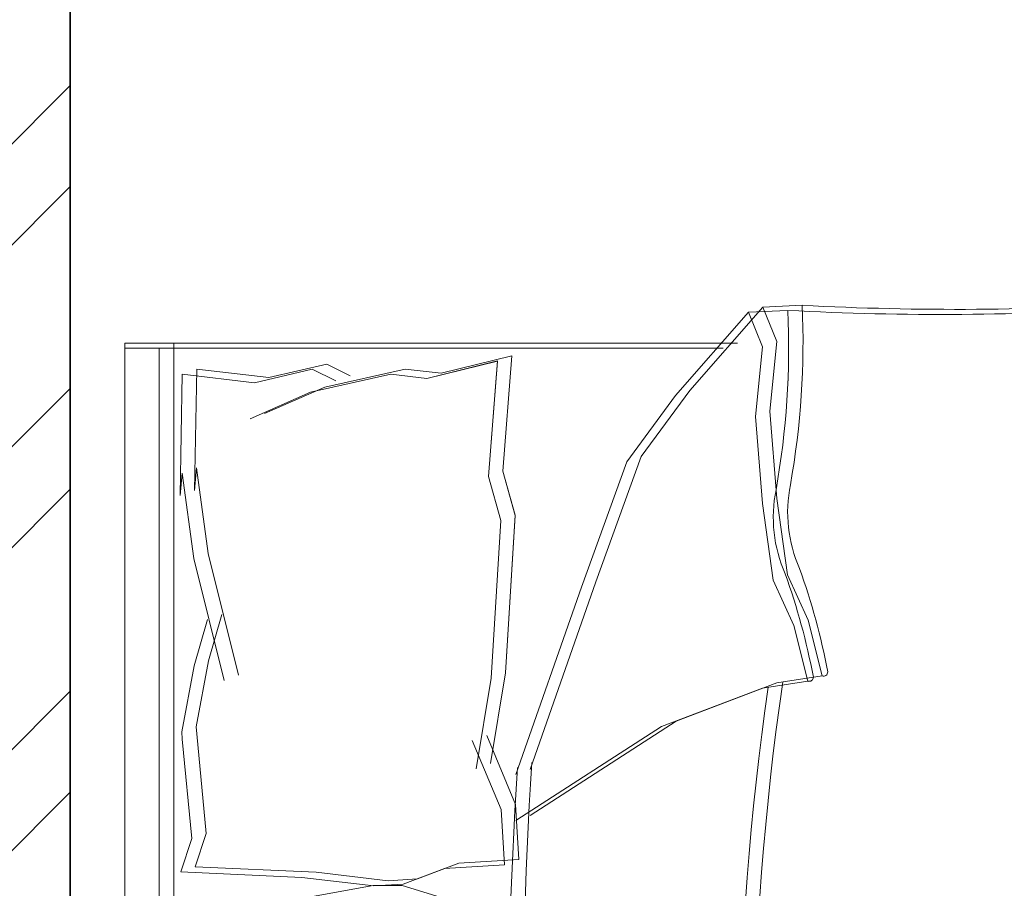
# Model space of a CAD drawing. Units: inches. Extents: x 2168 to 3056, y 1130 to 2629.
# Tile 27 of 42: x 2462 to 2505, y 2347 to 2386. Entities that reach past the tile are written whole.
import ezdxf

# ---------------------------------------------------------------- set-up
doc = ezdxf.new("R2010")
doc.units = ezdxf.units.IN
doc.layers.add('A-FURN', color=8, linetype='Continuous', lineweight=13)
doc.layers.add('A-WALL', color=7, linetype='Continuous', lineweight=35)
doc.layers.add('A-WALL-PATT', color=143, linetype='Continuous', lineweight=13, true_color=0x7aafdf)

# ---------------------------------------------------------------- blocks, each defined once
blk = doc.blocks.new('BED-DOUBLE')
for p, q in [((28.385, 53.096), (25.135, 49.391)), ((28.385, 53.096), (25.135, 49.391)), ((30.13, 53.176), (28.385, 53.096, 3.871)), ((30.13, 53.175), (28.385, 53.096, 3.871)), ((29.005, 51.559), (28.385, 53.096)), ((29.005, 51.559), (28.385, 53.096)), ((27.746, 52.868), (24.496, 49.162)), ((27.746, 52.868), (24.496, 49.162)), ((29.491, 52.947), (27.746, 52.868, 3.871)), ((29.491, 52.947), (27.746, 52.868, 3.871)), ((28.365, 51.331), (27.746, 52.868)), ((28.365, 51.33), (27.746, 52.868)), ((0, 51.494), (0.64, 51.494)), ((0, 3.475), (0, 51.494)), ((0, 51.266), (26.61, 51.266)), ((0, 51.265), (26.61, 51.265)), ((0.64, 51.494), (27.249, 51.494)), ((0.64, 51.494), (27.249, 51.494)), ((1.534, 3.475), (1.534, 51.266)), ((1.534, 3.475), (1.534, 51.265)), ((2.173, 3.704), (2.173, 51.494)), ((2.173, 3.703), (2.173, 51.494)), ((28.056, 48.233), (28.365, 51.331)), ((28.056, 48.233), (28.365, 51.33)), ((28.695, 48.462), (29.005, 51.559)), ((28.695, 48.461), (29.005, 51.559)), ((17.212, 50.927), (14.074, 50.151)), ((17.212, 50.927), (14.074, 50.151)), ((16.809, 45.795), (17.212, 50.927)), ((16.809, 45.795), (17.212, 50.927)), ((6.407, 49.962), (8.978, 50.557)), ((6.407, 49.962), (8.978, 50.557)), ((8.978, 50.557), (10.024, 50.043)), ((8.978, 50.557), (10.024, 50.043)), ((16.573, 50.699), (13.434, 49.923)), ((16.573, 50.698), (13.434, 49.923)), ((16.169, 45.567), (16.573, 50.699)), ((16.169, 45.566), (16.573, 50.698)), ((2.557, 50.112), (2.46, 44.71)), ((2.557, 50.112), (2.46, 44.71)), ((2.557, 50.112), (5.768, 49.734)), ((2.557, 50.112), (5.768, 49.733)), ((3.197, 50.341), (3.1, 44.938)), ((3.197, 50.34), (3.1, 44.938)), ((3.197, 50.341), (6.407, 49.962)), ((3.197, 50.34), (6.407, 49.962)), ((5.768, 49.734), (8.339, 50.329)), ((5.768, 49.733), (8.339, 50.328)), ((11.829, 50.112), (8.257, 49.31)), ((11.829, 50.112), (8.257, 49.309)), ((8.339, 50.329), (9.385, 49.815)), ((8.339, 50.328), (9.385, 49.814)), ((12.468, 50.341), (8.897, 49.538)), ((12.468, 50.34), (8.897, 49.538)), ((13.434, 49.923), (11.829, 50.112)), ((13.434, 49.923), (11.829, 50.112)), ((14.074, 50.151), (12.468, 50.341)), ((14.074, 50.151), (12.468, 50.34)), ((8.897, 49.538), (6.218, 48.357)), ((8.897, 49.538), (6.218, 48.357)), ((8.257, 49.31), (5.579, 48.128)), ((8.257, 49.309), (5.579, 48.128)), ((24.496, 49.162), (22.329, 46.22)), ((24.496, 49.162), (22.329, 46.22)), ((25.135, 49.391), (22.968, 46.448)), ((25.135, 49.391), (22.968, 46.448)), ((28.365, 44.361), (28.056, 48.233)), ((28.365, 44.361), (28.056, 48.233)), ((29.005, 44.59), (28.695, 48.462)), ((29.005, 44.589), (28.695, 48.461)), ((22.968, 46.448), (20.956, 40.873)), ((22.968, 46.448), (20.956, 40.873)), ((22.329, 46.22), (20.317, 40.644)), ((22.329, 46.22), (20.317, 40.644)), ((2.46, 44.71), (2.543, 45.713)), ((2.46, 44.71), (2.543, 45.712)), ((2.543, 45.713), (3.07, 41.915)), ((2.543, 45.712), (3.07, 41.914)), ((3.1, 44.938), (3.182, 45.941)), ((3.1, 44.938), (3.182, 45.941)), ((3.182, 45.941), (3.709, 42.143)), ((3.182, 45.941), (3.709, 42.143)), ((16.727, 43.606), (16.169, 45.567)), ((16.727, 43.606), (16.169, 45.566)), ((17.366, 43.835), (16.809, 45.795)), ((17.366, 43.834), (16.809, 45.795)), ((28.83, 40.954), (28.365, 44.361)), ((28.83, 40.954), (28.365, 44.361)), ((29.469, 41.183), (29.005, 44.59)), ((29.469, 41.182), (29.005, 44.589)), ((16.935, 36.825), (17.366, 43.835)), ((16.935, 36.824), (17.366, 43.834)), ((16.295, 36.596), (16.727, 43.606)), ((16.295, 36.596), (16.727, 43.606)), ((3.709, 42.143), (5.062, 36.724)), ((3.709, 42.143), (5.062, 36.723)), ((3.07, 41.915), (4.422, 36.495)), ((3.07, 41.914), (4.422, 36.495)), ((30.398, 39.169), (29.469, 41.183)), ((30.398, 39.169), (29.469, 41.182)), ((20.956, 40.873), (18.023, 32.535)), ((20.956, 40.873), (18.023, 32.534)), ((29.758, 38.941), (28.83, 40.954)), ((29.758, 38.941), (28.83, 40.954)), ((20.317, 40.644), (17.384, 32.306)), ((20.317, 40.644), (17.384, 32.306)), ((4.313, 39.429), (3.718, 37.364)), ((4.313, 39.429), (3.718, 37.364)), ((3.674, 39.2), (3.079, 37.136)), ((3.674, 39.2), (3.079, 37.135)), ((31.017, 36.691), (30.398, 39.169)), ((31.017, 36.691), (30.398, 39.169)), ((30.377, 36.463), (29.758, 38.941)), ((30.377, 36.463), (29.758, 38.941)), ((3.718, 37.364), (3.177, 34.433)), ((3.718, 37.364), (3.177, 34.433)), ((3.079, 37.136), (2.537, 34.205)), ((3.079, 37.135), (2.537, 34.205)), ((16.268, 32.793), (16.935, 36.825)), ((16.268, 32.793), (16.935, 36.824)), ((15.629, 32.564), (16.295, 36.596)), ((15.629, 32.564), (16.295, 36.596)), ((24.516, 34.678), (29.005, 36.381)), ((24.516, 34.678), (29.005, 36.381)), ((28.365, 36.153), (30.377, 36.463)), ((28.365, 36.153), (30.377, 36.463)), ((29.005, 36.381), (31.017, 36.691)), ((29.005, 36.381), (31.017, 36.691)), ((23.877, 34.45), (28.365, 36.153)), ((23.877, 34.449), (28.365, 36.153)), ((18.023, 30.488), (24.516, 34.678)), ((18.023, 30.488), (24.516, 34.678)), ((2.537, 34.205), (2.557, 33.884)), ((2.537, 34.205), (2.557, 33.884)), ((3.177, 34.433), (3.197, 34.112)), ((3.177, 34.433), (3.197, 34.112)), ((17.384, 30.259), (23.877, 34.45)), ((17.384, 30.259), (23.877, 34.449)), ((2.557, 33.884), (2.979, 29.456)), ((2.557, 33.884), (2.979, 29.456)), ((3.197, 34.112), (3.618, 29.684)), ((3.197, 34.112), (3.618, 29.684)), ((16.74, 30.751), (15.455, 33.821)), ((16.74, 30.75), (15.455, 33.821)), ((17.379, 30.979), (16.094, 34.049)), ((17.379, 30.979), (16.094, 34.049)), ((16.893, 28.298), (16.74, 30.751)), ((16.893, 28.298), (16.74, 30.75)), ((17.532, 28.526), (17.379, 30.979)), ((17.532, 28.526), (17.379, 30.979)), ((2.979, 29.456), (2.492, 27.977)), ((2.979, 29.456), (2.492, 27.977)), ((3.618, 29.684), (3.131, 28.206)), ((3.618, 29.684), (3.131, 28.205)), ((14.856, 28.359), (17.532, 28.526)), ((14.856, 28.359), (17.532, 28.526)), ((3.131, 28.206), (8.507, 27.962)), ((3.131, 28.205), (8.507, 27.962)), ((12.377, 27.436), (14.217, 28.131)), ((12.377, 27.436), (14.217, 28.13)), ((13.016, 27.665), (14.856, 28.359)), ((13.016, 27.664), (14.856, 28.359)), ((14.217, 28.131), (16.893, 28.298)), ((14.217, 28.13), (16.893, 28.298)), ((2.492, 27.977), (7.867, 27.734)), ((2.492, 27.977), (7.867, 27.733)), ((7.867, 27.734), (11.078, 27.355)), ((7.867, 27.733), (11.078, 27.355)), ((8.507, 27.962), (11.718, 27.583)), ((8.507, 27.962), (11.718, 27.583)), ((11.718, 27.583), (13.016, 27.665)), ((11.718, 27.583), (13.016, 27.664)), ((7.86, 26.789), (11.04, 27.368)), ((7.86, 26.789), (11.04, 27.367)), ((11.04, 27.368), (12.342, 27.368)), ((11.04, 27.367), (12.342, 27.367)), ((11.078, 27.355), (12.377, 27.436)), ((11.078, 27.355), (12.377, 27.436)), ((12.342, 27.368), (14.221, 26.789)), ((12.342, 27.367), (14.221, 26.789))]:
    blk.add_line(p, q)
for centre, radius, start, end in [((36.315, 182.266), 129.499, 266.97912, 273.83645), ((36.315, 182.266), 129.499, 266.97912, 273.83645), ((-6.017, 51.556), 36.183, 349.8763, 2.5657), ((-6.017, 51.556), 36.183, 349.8763, 2.5657), ((36.955, 182.494), 129.499, 266.97912, 273.83645), ((36.955, 182.494), 129.499, 266.97912, 273.83645), ((-6.656, 51.328), 36.183, 349.8763, 2.5657), ((-6.656, 51.327), 36.183, 349.8763, 2.5657), ((35.706, 43.972), 6.224, 168.6608, 203.7384), ((35.706, 43.972), 6.224, 168.6608, 203.7384), ((35.067, 43.744), 6.224, 168.6608, 203.7384), ((35.067, 43.743), 6.224, 168.6608, 203.7384), ((1.482, 31.154), 29.654, 10.6617, 19.8806), ((1.482, 31.154), 29.654, 10.6617, 19.8806), ((2.122, 31.382), 29.654, 10.6617, 19.8806), ((2.122, 31.382), 29.654, 10.6617, 19.8806), ((31.079, 36.865), 0.185, 250.2464, 1.1377), ((31.079, 36.865), 0.185, 250.2464, 1.1377), ((156.956, 17.984), 129.02, 171.78449, 186.90062), ((156.956, 17.984), 129.02, 171.78449, 186.90062), ((30.44, 36.637), 0.185, 250.2464, 1.1377), ((30.44, 36.636), 0.185, 250.2464, 1.1377), ((156.317, 17.756), 129.02, 171.78449, 186.90062), ((156.317, 17.756), 129.02, 171.78449, 186.90062), ((182.053, 21.359), 164.969, 176.08655, 186.78213), ((182.053, 21.359), 164.969, 176.08655, 186.78213), ((182.692, 21.587), 164.969, 176.08655, 186.78213), ((182.692, 21.587), 164.969, 176.08655, 186.78213)]:
    blk.add_arc(centre, radius, start, end)

msp = doc.modelspace()

# ---------------------------------------------------------------- hatches: boundary and pattern name
at = {"layer": 'A-WALL-PATT'}
h = msp.add_hatch(dxfattribs=at)
h.set_pattern_fill('ANSI32', color=256)
h.paths.add_polyline_path([(2463.796, 2409.389), (2467.387, 2409.389), (2467.387, 2413.889), (2454.768, 2413.889), (2454.768, 2411.639), (2454.768, 2409.389), (2459.296, 2409.389), (2459.296, 2265.389), (2455.644, 2265.389), (2455.644, 2260.889), (2467.349, 2260.889), (2467.349, 2263.139), (2467.349, 2265.389), (2463.796, 2265.389)])
h.paths.add_polyline_path([(2431.596, 2413.889), (2409.647, 2413.889), (2409.647, 2409.389), (2431.596, 2409.389), (2431.596, 2411.639)])
h.paths.add_polyline_path([(2349.647, 2413.889), (2331.796, 2413.889), (2331.796, 2362.671), (2336.296, 2362.671), (2336.296, 2409.389), (2349.647, 2409.389), (2349.647, 2411.639)])
h.paths.add_polyline_path([(2634.149, 2411.639), (2634.149, 2413.889), (2562.293, 2413.889), (2562.293, 2409.389), (2595.796, 2409.389), (2595.796, 2280.309), (2595.826, 2280.309), (2595.826, 2265.389), (2499.91, 2265.389), (2499.91, 2260.889), (2550.796, 2260.889), (2550.796, 2117.308), (2555.296, 2117.308), (2555.296, 2168.08), (2571.93, 2168.08), (2571.93, 2176.889), (2559.796, 2176.889), (2559.796, 2256.389), (2640.796, 2256.389), (2640.796, 2176.889), (2626.428, 2176.889), (2626.428, 2168.08), (2645.296, 2168.08), (2645.296, 2116.637), (2649.796, 2116.637), (2649.796, 2260.889), (2691.251, 2260.889), (2691.251, 2263.139), (2691.251, 2265.389), (2670.655, 2265.389), (2670.655, 2265.365), (2600.296, 2265.365), (2600.296, 2280.258), (2600.296, 2409.389), (2634.149, 2409.389)])
h.paths.add_polyline_path([(2600.296, 2473.889), (2612.84, 2473.889), (2612.84, 2478.389), (2572.636, 2478.389), (2572.636, 2473.889), (2595.796, 2473.889), (2595.796, 2413.889), (2600.296, 2413.889)])
h.paths.add_polyline_path([(2535.796, 2473.889), (2548.636, 2473.889), (2548.636, 2478.389), (2531.396, 2478.389), (2531.396, 2413.889), (2521.6, 2413.889), (2521.6, 2409.389), (2539.239, 2409.389), (2539.239, 2411.639), (2539.239, 2413.889), (2535.796, 2413.889)])
h.paths.add_polyline_path([(2664.796, 2478.389), (2636.84, 2478.389), (2636.84, 2473.889), (2660.296, 2473.889), (2660.296, 2413.889), (2656.165, 2413.889), (2656.165, 2409.389), (2671.684, 2409.389), (2671.684, 2411.639), (2671.684, 2413.889), (2664.796, 2413.889)])
h.paths.add_polyline_path([(2705.942, 2413.889), (2695.684, 2413.889), (2695.684, 2409.389), (2705.942, 2409.389)])
h.paths.add_polyline_path([(2741.35, 2413.889), (2728.733, 2413.889), (2728.733, 2411.639), (2728.733, 2409.389), (2732.296, 2409.389), (2732.296, 2265.389), (2725.733, 2265.389), (2725.733, 2260.889), (2740.917, 2260.889), (2740.917, 2263.139), (2740.917, 2265.389), (2736.796, 2265.389), (2736.796, 2409.389), (2741.35, 2409.389)])
h.paths.add_polyline_path([(2785.655, 2413.889), (2764.546, 2413.889), (2764.486, 2409.389), (2785.655, 2409.389), (2785.655, 2411.639)])
h.paths.add_polyline_path([(2864.296, 2413.889), (2845.655, 2413.889), (2845.655, 2409.389), (2859.796, 2409.389), (2859.796, 2368.425), (2864.296, 2368.425)])
h.paths.add_polyline_path([(2864.296, 2308.425), (2862.046, 2308.425), (2859.796, 2308.425), (2859.796, 2265.389), (2774.483, 2265.389), (2774.483, 2263.139), (2774.483, 2260.889), (2781.796, 2260.889), (2781.796, 2226.654), (2786.296, 2226.654), (2786.296, 2260.889), (2859.796, 2260.889), (2859.796, 2241.352), (2864.296, 2241.352)])
h.paths.add_polyline_path([(2864.296, 2217.352), (2862.046, 2217.352), (2859.796, 2217.352), (2859.796, 2200.889), (2786.296, 2200.889), (2786.296, 2205.931), (2784.046, 2205.931), (2781.796, 2205.931), (2781.796, 2150.974), (2786.296, 2150.974), (2786.296, 2161.889), (2859.796, 2161.889), (2859.796, 2144.419), (2864.296, 2144.419)])
h.paths.add_polyline_path([(2859.796, 2196.389), (2859.796, 2166.389), (2786.296, 2166.389), (2786.296, 2196.389)], flags=16)
h.paths.add_polyline_path([(2864.296, 2108.419), (2862.046, 2108.419), (2859.796, 2108.419), (2859.796, 2080.889), (2786.296, 2080.889), (2786.296, 2111.993), (2781.796, 2111.993), (2781.796, 2080.889), (2649.796, 2080.889), (2649.796, 2086.036), (2647.546, 2086.036), (2645.296, 2086.036), (2645.296, 2071.739), (2649.796, 2071.739), (2649.796, 2076.389), (2781.796, 2076.389), (2781.796, 2041.792), (2786.296, 2041.792), (2786.296, 2076.389), (2859.796, 2076.389), (2859.796, 2058.577), (2864.296, 2058.577)])
h.paths.add_polyline_path([(2864.296, 2022.577), (2859.796, 2022.577), (2859.796, 1992.389), (2786.296, 1992.389), (2786.296, 1999.573), (2781.796, 1999.573), (2781.796, 1848.085), (2784.046, 1848.085), (2786.296, 1848.085), (2786.296, 1851.389), (2859.796, 1851.389), (2859.796, 1838.258), (2864.296, 1838.258)], flags=17)
h.paths.add_polyline_path([(2859.796, 1987.889), (2859.796, 1855.889), (2786.296, 1855.889), (2786.296, 1987.889)], flags=16)
h.paths.add_polyline_path([(2823.046, 1987.889), (2841.421, 1921.889), (2823.046, 1855.889)], flags=0)
h.paths.add_polyline_path([(2864.296, 1814.258), (2859.796, 1814.258), (2859.796, 1791.389), (2786.296, 1791.389), (2786.296, 1825.658), (2784.046, 1825.658), (2781.796, 1825.658), (2781.796, 1791.389), (2720.155, 1791.389), (2720.155, 1791.265), (2649.796, 1791.265), (2649.796, 1806.159), (2649.796, 2038.983), (2647.546, 2038.983), (2645.296, 2038.983), (2645.296, 1783.925), (2649.796, 1783.925), (2649.796, 1786.889), (2781.796, 1786.889), (2781.796, 1746.789), (2786.296, 1746.789), (2786.296, 1786.889), (2859.796, 1786.889), (2859.796, 1770.083), (2864.296, 1770.083)])
h.paths.add_polyline_path([(2864.296, 1734.083), (2862.046, 1734.083), (2859.796, 1734.083), (2859.796, 1705.889), (2786.296, 1705.889), (2786.296, 1714.166), (2781.796, 1714.166), (2781.796, 1660.527), (2786.296, 1660.527), (2786.296, 1666.889), (2859.796, 1666.889), (2859.796, 1648.342), (2864.296, 1648.342)])
h.paths.add_polyline_path([(2786.296, 1701.389), (2859.796, 1701.389), (2859.796, 1671.389), (2786.296, 1671.389)], flags=16)
h.paths.add_polyline_path([(2649.796, 1756.576), (2647.546, 1756.576), (2645.296, 1756.576), (2645.296, 1606.889), (2555.296, 1606.889), (2555.296, 1749.513), (2553.046, 1749.513), (2550.796, 1749.513), (2550.796, 1606.889), (2503.006, 1606.889), (2503.006, 1604.639), (2503.006, 1602.389), (2595.796, 1602.389), (2595.849, 1602.389), (2595.849, 1587.495), (2595.796, 1458.389), (2561.502, 1458.389), (2561.502, 1456.139), (2561.502, 1453.889), (2595.796, 1453.889), (2595.796, 1381.889), (2573.438, 1381.889), (2573.438, 1377.389), (2613.01, 1377.389), (2613.01, 1379.639), (2613.01, 1381.889), (2600.296, 1381.889), (2600.296, 1453.889), (2634.327, 1453.889), (2634.327, 1458.389), (2600.296, 1458.389), (2600.296, 1602.389), (2670.655, 1602.389), (2694.095, 1602.389), (2694.095, 1606.889), (2649.796, 1606.889)])
h.paths.add_polyline_path([(2736.796, 1602.389), (2741.562, 1602.389), (2741.562, 1606.889), (2726.203, 1606.889), (2726.203, 1604.639), (2726.203, 1602.389), (2732.296, 1602.389), (2732.296, 1458.389), (2727.899, 1458.389), (2727.899, 1453.889), (2740.821, 1453.889), (2740.821, 1456.139), (2740.821, 1458.389), (2736.796, 1458.389)])
h.paths.add_polyline_path([(2859.796, 1606.889), (2786.296, 1606.889), (2786.296, 1637.334), (2784.046, 1637.334), (2781.796, 1637.334), (2781.796, 1606.889), (2775.612, 1606.889), (2775.612, 1602.389), (2859.796, 1602.389)])
h.paths.add_polyline_path([(2864.296, 1624.342), (2862.046, 1624.342), (2859.796, 1624.342), (2859.796, 1570.39), (2864.296, 1570.39)])
h.paths.add_polyline_path([(2864.296, 1510.39), (2862.046, 1510.39), (2859.796, 1510.39), (2859.796, 1458.389), (2846.735, 1458.389), (2846.735, 1456.139), (2846.735, 1453.889), (2864.296, 1453.889)])
h.paths.add_polyline_path([(2786.735, 1458.389), (2765.444, 1458.389), (2765.444, 1453.889), (2786.735, 1453.889)])
h.paths.add_polyline_path([(2706.004, 1458.389), (2695.36, 1458.389), (2695.36, 1453.889), (2706.004, 1453.889), (2706.004, 1456.139)])
h.paths.add_polyline_path([(2671.36, 1456.139), (2671.36, 1458.389), (2655.986, 1458.389), (2655.986, 1456.139), (2655.986, 1453.889), (2660.296, 1453.889), (2660.296, 1381.889), (2637.01, 1381.889), (2637.01, 1377.389), (2664.796, 1377.389), (2664.796, 1453.889), (2671.36, 1453.889)], flags=17)
h.paths.add_polyline_path([(2539.829, 1458.389), (2520.237, 1458.389), (2520.237, 1453.889), (2531.296, 1453.889), (2531.296, 1377.389), (2546.449, 1377.389), (2546.449, 1379.639), (2546.449, 1381.889), (2535.796, 1381.889), (2535.796, 1453.889), (2539.829, 1453.889)], flags=17)
h.paths.add_polyline_path([(2496.237, 1458.389), (2489.13, 1458.389), (2489.13, 1453.889), (2496.237, 1453.889), (2496.237, 1456.139)])
h.paths.add_polyline_path([(2467.433, 1456.139), (2467.433, 1458.389), (2463.796, 1458.389), (2463.796, 1602.389), (2468.242, 1602.389), (2468.242, 1605.7), (2468.242, 1606.889), (2454.602, 1606.889), (2454.602, 1602.389), (2459.296, 1602.389), (2459.296, 1458.389), (2454.24, 1458.389), (2454.24, 1453.889), (2467.433, 1453.889)])
h.paths.add_polyline_path([(2431.601, 1456.139), (2431.601, 1458.389), (2411.386, 1458.389), (2411.386, 1453.889), (2431.601, 1453.889)])
h.paths.add_polyline_path([(2351.386, 1458.389), (2336.296, 1458.389), (2336.296, 1490.693), (2334.046, 1490.693), (2331.796, 1490.693), (2331.796, 1453.889), (2351.386, 1453.889), (2351.386, 1456.139)])
h.paths.add_polyline_path([(2336.296, 1629.705), (2331.796, 1629.705), (2331.796, 1552.317), (2336.296, 1552.317), (2336.296, 1602.389), (2406.655, 1602.389), (2423.472, 1602.389), (2423.472, 1606.889), (2418.796, 1606.889), (2418.796, 1643.678), (2416.546, 1643.678), (2414.296, 1643.678), (2414.296, 1606.889), (2336.296, 1606.889)])
h.paths.add_polyline_path([(2418.796, 1714.384), (2414.296, 1714.384), (2414.296, 1705.889), (2336.296, 1705.889), (2336.296, 1731.324), (2334.046, 1731.324), (2331.796, 1731.324), (2331.796, 1653.705), (2334.046, 1653.705), (2336.296, 1653.705), (2336.296, 1666.889), (2414.296, 1666.889), (2414.296, 1663.589), (2418.796, 1663.589)])
h.paths.add_polyline_path([(2336.296, 1701.389), (2414.296, 1701.389), (2414.296, 1671.389), (2336.296, 1671.389)], flags=16)
h.paths.add_polyline_path([(2555.296, 2040.059), (2550.796, 2040.059), (2550.796, 1791.389), (2550.561, 1791.205), (2480.202, 1791.205), (2418.796, 1791.389), (2418.796, 1825.448), (2416.546, 1825.448), (2414.296, 1825.448), (2414.296, 1791.389), (2336.296, 1791.389), (2336.296, 1806.409), (2331.796, 1806.409), (2331.796, 1767.324), (2336.296, 1767.324), (2336.296, 1786.889), (2414.296, 1786.889), (2414.296, 1745.457), (2418.796, 1745.457), (2418.796, 1786.889), (2550.796, 1786.889), (2550.796, 1783.011), (2555.296, 1783.011)])
h.paths.add_polyline_path([(2418.796, 1923.389), (2423.207, 1923.389), (2423.207, 1925.639), (2423.207, 1927.889), (2418.796, 1927.889), (2418.796, 2000.048), (2414.296, 2000.048), (2414.296, 1992.389), (2336.296, 1992.389), (2336.296, 1987.889), (2414.296, 1987.889), (2414.296, 1855.889), (2336.296, 1855.889), (2336.296, 1851.389), (2414.296, 1851.389), (2414.296, 1846.759), (2418.796, 1846.759)], flags=17)
h.paths.add_polyline_path([(2336.296, 2019.294), (2334.046, 2019.294), (2331.796, 2019.294), (2331.796, 1830.409), (2336.296, 1830.409)], flags=17)
h.paths.add_polyline_path([(2550.796, 1927.889), (2453.541, 1927.889), (2453.541, 1925.639), (2453.541, 1923.389), (2550.796, 1923.389)], flags=17)
h.paths.add_polyline_path([(2744.987, 1927.889), (2649.796, 1927.889), (2649.796, 1923.389), (2744.987, 1923.389), (2744.987, 1925.639)], flags=17)
h.paths.add_polyline_path([(2555.296, 2086.458), (2553.046, 2086.458), (2550.796, 2086.458), (2550.796, 2080.889), (2418.796, 2080.889), (2336.296, 2080.889), (2336.296, 2115.399), (2334.046, 2115.399), (2331.796, 2115.399), (2331.796, 2055.294), (2336.296, 2055.294), (2336.296, 2076.389), (2550.796, 2076.389), (2550.796, 2071.538), (2555.296, 2071.538)])
h.paths.add_polyline_path([(2418.796, 2121.389), (2414.296, 2121.389), (2414.296, 2080.889), (2418.796, 2080.889)])
h.paths.add_polyline_path([(2418.796, 2076.389), (2414.296, 2076.389), (2414.296, 2035.123), (2418.796, 2035.123)])
h.paths.add_polyline_path([(2422.868, 2263.139), (2422.868, 2265.389), (2406.655, 2265.389), (2406.655, 2265.359), (2336.296, 2265.359), (2336.296, 2280.252), (2336.296, 2302.671), (2334.046, 2302.671), (2331.796, 2302.671), (2331.796, 2246.853), (2336.296, 2246.853), (2336.296, 2260.889), (2414.296, 2260.889), (2414.296, 2223.996), (2418.796, 2223.996), (2418.796, 2260.889), (2422.868, 2260.889)])
h.paths.add_polyline_path([(2418.796, 2204.783), (2416.546, 2204.783), (2414.296, 2204.783), (2414.296, 2200.889), (2336.296, 2200.889), (2336.296, 2220.853), (2331.796, 2220.853), (2331.796, 2151.399), (2336.296, 2151.399), (2336.296, 2161.889), (2414.296, 2161.889), (2414.296, 2153.726), (2418.796, 2153.726)])
h.paths.add_polyline_path([(2414.296, 2196.389), (2414.296, 2166.389), (2336.296, 2166.389), (2336.296, 2196.389)], flags=16)
h.paths.add_polyline_path([(2375.296, 2181.389), (2336.296, 2166.389), (2336.296, 2196.389)], flags=0)
h.paths.add_polyline_path([(2809.595, 2172.34), (2838.804, 2172.34), (2838.804, 2190.997), (2809.595, 2190.997)], flags=8)
h.paths.add_polyline_path([(2849.75, 1919.585), (2849.75, 1952.672), (2831.093, 1952.672), (2831.093, 1919.585)], flags=8)
h.paths.add_polyline_path([(2808.875, 1901.967), (2808.875, 1937.85), (2790.149, 1937.85), (2790.149, 1901.967)], flags=8)
h.paths.add_polyline_path([(2806.285, 1671.896), (2835.493, 1671.896), (2835.493, 1690.553), (2806.285, 1690.553)], flags=8)
h.paths.add_polyline_path([(2353.186, 1676.549), (2382.395, 1676.549), (2382.395, 1695.207), (2353.186, 1695.207)], flags=8)
h.paths.add_polyline_path([(2360.083, 1832.308), (2389.241, 1832.308), (2389.241, 1850.966), (2360.083, 1850.966)], flags=25)
h.paths.add_polyline_path([(2354.822, 2167.823), (2384.031, 2167.823), (2384.031, 2186.481), (2354.822, 2186.481)], flags=8)

# ---------------------------------------------------------------- linework, layer by layer
at = {"layer": 'A-WALL'}
msp.add_line((2463.796, 2409.389), (2463.796, 2265.389), dxfattribs=at)

# ---------------------------------------------------------------- block references
at = {"layer": 'A-FURN'}
msp.add_blockref('BED-DOUBLE', (2466.223, 2320.021), dxfattribs=at)

doc.saveas('drawing.dxf')
